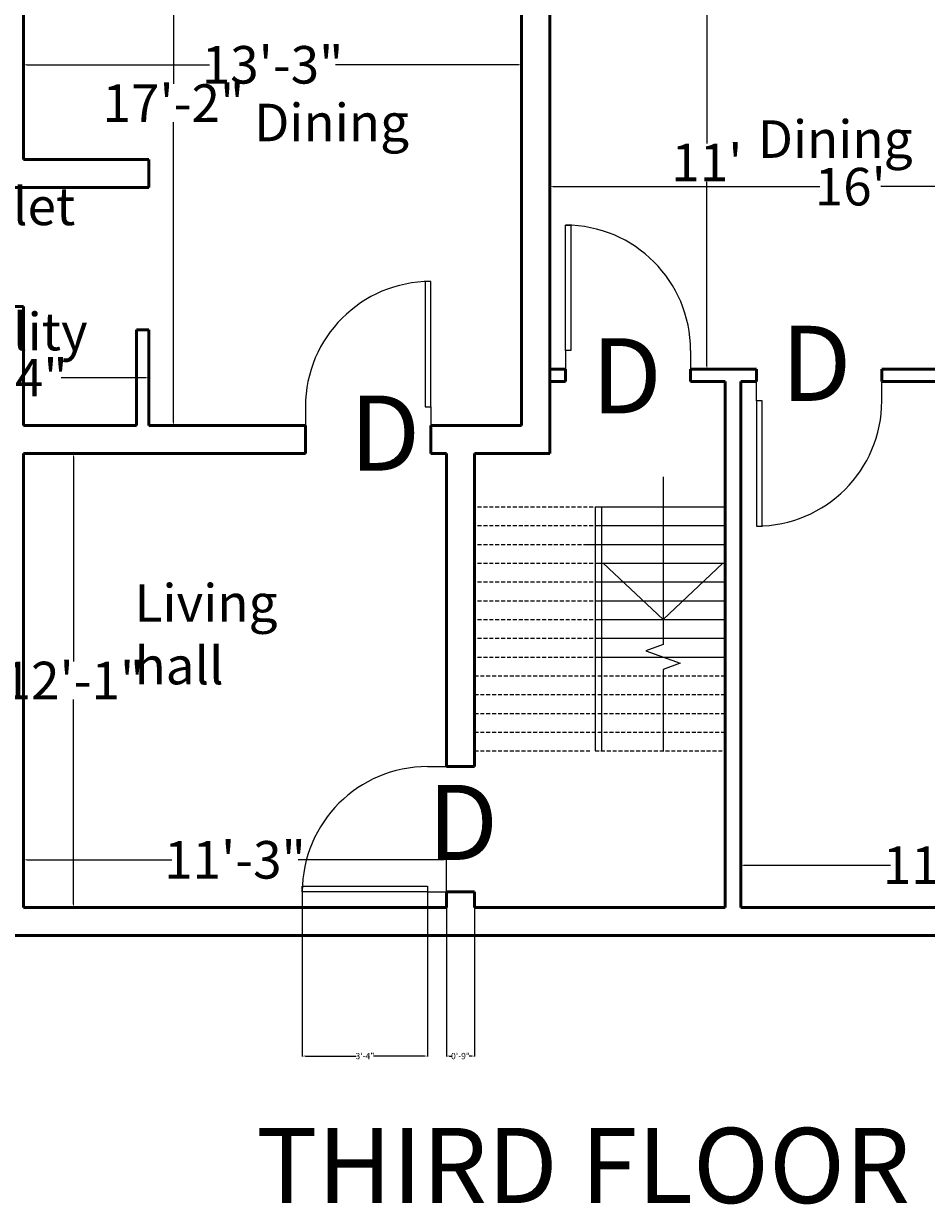
# Model space of a CAD drawing. Units: inches. Extents: x 409 to 7572, y 7 to 725.
# Tile 22 of 38: x 4335 to 4623, y 71 to 448. Entities that reach past the tile are written whole.
import ezdxf

# ---------------------------------------------------------------- set-up
doc = ezdxf.new("R2010")
doc.units = ezdxf.units.IN
doc.header["$MEASUREMENT"] = 0
doc.linetypes.add('HIDDEN', pattern=[0.375, 0.25, -0.125])
for name, color, linetype, lineweight in [('A-ANNO-DIMS', 2, 'Continuous', 18), ('A-ANNO-SYMB', 3, 'Continuous', 25), ('A-ANNO-TEXT', 7, 'Continuous', 35), ('A-AREA-IDEN', 7, 'Continuous', 25), ('A-DOOR', 3, 'Continuous', 25), ('A-FLOR-STRS', 6, 'Continuous', 25), ('A-FLOR-STRS-OVHD', 6, 'HIDDEN', 18), ('A-WALL', 7, 'Continuous', 50)]:
    doc.layers.add(name, color=color, linetype=linetype, lineweight=lineweight)
doc.styles.get("Standard").update_dxf_attribs({"font": 'arial.ttf'})
doc.dimstyles.get("Standard").update_dxf_attribs({"dimtxt": 2, "dimasz": 1, "dimexe": 0.18, "dimexo": 0.0625, "dimgap": 0.09, "dimtad": 0, "dimtih": 1, "dimtoh": 1, "dimdec": 0, "dimzin": 0, "dimdsep": 46, "dimlunit": 3, "dimtxsty": 'Standard', "dimcen": 0.09, "dimadec": 0, "dimazin": 0, "dimtfac": 1, "dimtdec": 0, "dimtofl": 0, "dimtmove": 0, "dimatfit": 3, "dimfxl": 1, "dimtolj": 1, "dimtzin": 0, "dimarcsym": 0})

# ---------------------------------------------------------------- blocks, each defined once
blk = doc.blocks.new('*U2')
for p, q in [((0, 0), (0, -6)), ((-40, 0), (-40, -6))]:
    blk.add_line(p, q)
blk.add_lwpolyline([(0, 0), (0, 40), (-1.75, 40), (-1.75, 0)], close=True)
blk.add_arc((0, 0), 40, 90, 180)
blk = doc.blocks.new('*U3')
for p, q in [((0, 0), (0, -6)), ((40, 0), (40, -6))]:
    blk.add_line(p, q)
blk.add_lwpolyline([(0, 0), (0, 40), (1.75, 40), (1.75, 0)], close=True)
blk.add_arc((0, 0), 40, 0, 90)
blk = doc.blocks.new('*U4')
for p, q in [((0, 0), (0, -6)), ((40, 0), (40, -6))]:
    blk.add_line(p, q)
blk.add_lwpolyline([(0, 0), (0, 40), (1.75, 40), (1.75, 0)], close=True)
blk.add_arc((0, 0), 40, 0, 90)
blk = doc.blocks.new('*U5')
for p, q in [((0, 0), (0, 6)), ((40, 0), (40, 6))]:
    blk.add_line(p, q)
blk.add_lwpolyline([(0, 0), (0, -40), (1.75, -40), (1.75, 0)], close=True)
blk.add_arc((0, 0), 40, 270, 0)
blk = doc.blocks.new('*D96')
at = {"layer": 'A-ANNO-DIMS', "color": 0, "lineweight": -2, "transparency": 16777216}
for p, q in [((4563.94, 165.59), (4563.94, 179.18)), ((4564.94, 179), (4611.8, 179)), ((4698.94, 179), (4652.08, 179)), ((4699.94, 165.59), (4699.94, 179.18))]:
    blk.add_line(p, q, dxfattribs=at)
at = {"layer": 'A-ANNO-DIMS', "color": 0, "transparency": 16777216}
for points in [[(4564.94, 179.16), (4564.94, 178.83), (4563.94, 179)], [(4698.94, 179.16), (4698.94, 178.83), (4699.94, 179)]]:
    blk.add_solid(points, dxfattribs=at)
at = {"layer": 'DEFPOINTS', "color": 0, "transparency": 16777216}
for p in [(4699.94, 179), (4563.94, 165.53), (4699.94, 165.53)]:
    blk.add_point(p, dxfattribs=at)
at = {"layer": 'A-ANNO-DIMS', "color": 0, "transparency": 16777216, "insert": (4631.94, 179), "char_height": 2, "attachment_point": 5}
blk.add_mtext('\\A1;{\\H6x;11\'-4"}', dxfattribs=at)
blk = doc.blocks.new('*D97')
at = {"layer": 'A-ANNO-DIMS', "color": 0, "lineweight": -2, "transparency": 16777216}
for p, q in [((4334.94, 165.59), (4334.94, 180.91)), ((4335.94, 180.73), (4382.3, 180.73)), ((4468.94, 180.73), (4422.58, 180.73)), ((4469.94, 165.59), (4469.94, 180.91))]:
    blk.add_line(p, q, dxfattribs=at)
at = {"layer": 'A-ANNO-DIMS', "color": 0, "transparency": 16777216}
for points in [[(4335.94, 180.9), (4335.94, 180.56), (4334.94, 180.73)], [(4468.94, 180.9), (4468.94, 180.56), (4469.94, 180.73)]]:
    blk.add_solid(points, dxfattribs=at)
at = {"layer": 'DEFPOINTS', "color": 0, "transparency": 16777216}
for p in [(4469.94, 180.73), (4334.94, 165.53), (4469.94, 165.53)]:
    blk.add_point(p, dxfattribs=at)
at = {"layer": 'A-ANNO-DIMS', "color": 0, "transparency": 16777216, "insert": (4402.44, 180.73), "char_height": 2, "attachment_point": 5}
blk.add_mtext('\\A1;{\\H6x;11\'-3"}', dxfattribs=at)
blk = doc.blocks.new('*D98')
at = {"layer": 'A-ANNO-DIMS', "color": 0, "lineweight": -2, "transparency": 16777216}
for p, q in [((4335, 310.53), (4351.04, 310.53)), ((4350.86, 309.53), (4350.86, 244.15)), ((4350.86, 166.53), (4350.86, 231.92)), ((4335, 165.53), (4351.04, 165.53))]:
    blk.add_line(p, q, dxfattribs=at)
at = {"layer": 'A-ANNO-DIMS', "color": 0, "transparency": 16777216}
for points in [[(4350.7, 309.53), (4351.03, 309.53), (4350.86, 310.53)], [(4350.7, 166.53), (4351.03, 166.53), (4350.86, 165.53)]]:
    blk.add_solid(points, dxfattribs=at)
at = {"layer": 'DEFPOINTS', "color": 0, "transparency": 16777216}
for p in [(4334.94, 310.53), (4334.94, 165.53), (4350.86, 165.53)]:
    blk.add_point(p, dxfattribs=at)
at = {"layer": 'A-ANNO-DIMS', "color": 0, "transparency": 16777216, "insert": (4350.86, 238.03), "char_height": 2, "attachment_point": 5}
blk.add_mtext('\\A1;{\\H6x;12\'-1"}', dxfattribs=at)
blk = doc.blocks.new('*D110')
at = {"layer": 'A-ANNO-DIMS', "color": 0, "lineweight": -2, "transparency": 16777216}
for p, q in [((4334.94, 404.59), (4334.94, 434.95)), ((4335.94, 434.77), (4394.3, 434.77)), ((4492.94, 434.77), (4434.58, 434.77)), ((4493.94, 404.59), (4493.94, 434.95))]:
    blk.add_line(p, q, dxfattribs=at)
at = {"layer": 'A-ANNO-DIMS', "color": 0, "transparency": 16777216}
for points in [[(4335.94, 434.93), (4335.94, 434.6), (4334.94, 434.77)], [(4492.94, 434.93), (4492.94, 434.6), (4493.94, 434.77)]]:
    blk.add_solid(points, dxfattribs=at)
at = {"layer": 'DEFPOINTS', "color": 0, "transparency": 16777216}
for p in [(4493.94, 434.77), (4334.94, 404.53), (4493.94, 404.53)]:
    blk.add_point(p, dxfattribs=at)
at = {"layer": 'A-ANNO-DIMS', "color": 0, "transparency": 16777216, "insert": (4414.44, 434.77), "char_height": 2, "attachment_point": 5}
blk.add_mtext('\\A1;{\\H6x;13\'-3"}', dxfattribs=at)
blk = doc.blocks.new('*D111')
at = {"layer": 'A-ANNO-DIMS', "color": 0, "lineweight": -2, "transparency": 16777216}
for p, q in [((4391.88, 525.53), (4382.6, 525.53)), ((4382.78, 524.53), (4382.78, 428.65)), ((4382.78, 320.53), (4382.78, 416.42)), ((4399.88, 319.53), (4382.6, 319.53))]:
    blk.add_line(p, q, dxfattribs=at)
at = {"layer": 'A-ANNO-DIMS', "color": 0, "transparency": 16777216}
for points in [[(4382.61, 524.53), (4382.94, 524.53), (4382.78, 525.53)], [(4382.61, 320.53), (4382.94, 320.53), (4382.78, 319.53)]]:
    blk.add_solid(points, dxfattribs=at)
at = {"layer": 'DEFPOINTS', "color": 0, "transparency": 16777216}
for p in [(4391.94, 525.53), (4382.78, 319.53), (4399.94, 319.53)]:
    blk.add_point(p, dxfattribs=at)
at = {"layer": 'A-ANNO-DIMS', "color": 0, "transparency": 16777216, "insert": (4382.78, 422.53), "char_height": 2, "attachment_point": 5}
blk.add_mtext('\\A1;{\\H6x;17\'-2"}', dxfattribs=at)
blk = doc.blocks.new('*D108')
at = {"layer": 'A-ANNO-DIMS', "color": 0, "lineweight": -2, "transparency": 16777216}
for p, q in [((4502.94, 403.47), (4502.94, 395.65)), ((4694.94, 403.47), (4694.94, 395.65)), ((4503.94, 395.83), (4589.23, 395.83)), ((4693.94, 395.83), (4608.65, 395.83))]:
    blk.add_line(p, q, dxfattribs=at)
at = {"layer": 'A-ANNO-DIMS', "color": 0, "transparency": 16777216}
for points in [[(4503.94, 396), (4503.94, 395.66), (4502.94, 395.83)], [(4693.94, 396), (4693.94, 395.66), (4694.94, 395.83)]]:
    blk.add_solid(points, dxfattribs=at)
at = {"layer": 'DEFPOINTS', "color": 0, "transparency": 16777216}
for p in [(4502.94, 403.53), (4694.94, 403.53), (4694.94, 395.83)]:
    blk.add_point(p, dxfattribs=at)
at = {"layer": 'A-ANNO-DIMS', "color": 0, "transparency": 16777216, "insert": (4598.94, 395.83), "char_height": 2, "attachment_point": 5}
blk.add_mtext("\\A1;{\\H6x;16'}", dxfattribs=at)
blk = doc.blocks.new('*D112')
at = {"layer": 'A-ANNO-DIMS', "color": 0, "lineweight": -2, "transparency": 16777216}
for p, q in [((4557.2, 469.53), (4552.96, 469.53)), ((4553.14, 468.53), (4553.14, 409.65)), ((4553.14, 338.53), (4553.14, 397.42)), ((4558.38, 337.53), (4552.96, 337.53))]:
    blk.add_line(p, q, dxfattribs=at)
at = {"layer": 'A-ANNO-DIMS', "color": 0, "transparency": 16777216}
for points in [[(4552.97, 468.53), (4553.31, 468.53), (4553.14, 469.53)], [(4552.97, 338.53), (4553.31, 338.53), (4553.14, 337.53)]]:
    blk.add_solid(points, dxfattribs=at)
at = {"layer": 'DEFPOINTS', "color": 0, "transparency": 16777216}
for p in [(4557.27, 469.53), (4553.14, 337.53), (4558.44, 337.53)]:
    blk.add_point(p, dxfattribs=at)
at = {"layer": 'A-ANNO-DIMS', "color": 0, "transparency": 16777216, "insert": (4553.14, 403.53), "char_height": 2, "attachment_point": 5}
blk.add_mtext("\\A1;{\\H6x;11'}", dxfattribs=at)
blk = doc.blocks.new('*D117')
at = {"layer": 'A-ANNO-DIMS', "color": 0, "lineweight": -2, "transparency": 16777216}
for p, q in [((4286.94, 346.33), (4286.94, 334.6)), ((4374.94, 346.33), (4374.94, 334.6)), ((4287.94, 334.78), (4314.95, 334.78)), ((4373.94, 334.78), (4346.93, 334.78))]:
    blk.add_line(p, q, dxfattribs=at)
at = {"layer": 'A-ANNO-DIMS', "color": 0, "transparency": 16777216}
for points in [[(4287.94, 334.95), (4287.94, 334.61), (4286.94, 334.78)], [(4373.94, 334.95), (4373.94, 334.61), (4374.94, 334.78)]]:
    blk.add_solid(points, dxfattribs=at)
at = {"layer": 'DEFPOINTS', "color": 0, "transparency": 16777216}
for p in [(4286.94, 346.39), (4374.94, 346.39), (4374.94, 334.78)]:
    blk.add_point(p, dxfattribs=at)
at = {"layer": 'A-ANNO-DIMS', "color": 0, "transparency": 16777216, "insert": (4330.94, 334.78), "char_height": 2, "attachment_point": 5}
blk.add_mtext('\\A1;{\\H6x;7\'-4"}', dxfattribs=at)
blk = doc.blocks.new('*D189')
at = {"layer": 'A-ANNO-DIMS', "color": 0, "lineweight": -2, "transparency": 16777216}
for p, q in [((4469.94, 165.47), (4469.94, 117.85)), ((4478.94, 165.47), (4478.94, 117.85)), ((4470.94, 118.03), (4471.69, 118.03)), ((4477.94, 118.03), (4477.19, 118.03))]:
    blk.add_line(p, q, dxfattribs=at)
at = {"layer": 'A-ANNO-DIMS', "color": 0, "transparency": 16777216}
for points in [[(4470.94, 118.2), (4470.94, 117.86), (4469.94, 118.03)], [(4477.94, 118.2), (4477.94, 117.86), (4478.94, 118.03)]]:
    blk.add_solid(points, dxfattribs=at)
at = {"layer": 'DEFPOINTS', "color": 0, "transparency": 16777216}
for p in [(4469.94, 165.53), (4478.94, 165.53), (4478.94, 118.03)]:
    blk.add_point(p, dxfattribs=at)
at = {"layer": 'A-ANNO-DIMS', "color": 0, "transparency": 16777216, "insert": (4474.44, 118.03), "char_height": 2, "attachment_point": 5}
blk.add_mtext('\\A1;0\'-9"', dxfattribs=at)
blk = doc.blocks.new('*D191')
at = {"layer": 'A-ANNO-DIMS', "color": 0, "lineweight": -2, "transparency": 16777216}
for p, q in [((4423.94, 170.47), (4423.94, 117.85)), ((4463.94, 170.47), (4463.94, 117.85)), ((4424.94, 118.03), (4441.19, 118.03)), ((4462.94, 118.03), (4446.69, 118.03))]:
    blk.add_line(p, q, dxfattribs=at)
at = {"layer": 'A-ANNO-DIMS', "color": 0, "transparency": 16777216}
for points in [[(4424.94, 118.2), (4424.94, 117.86), (4423.94, 118.03)], [(4462.94, 118.2), (4462.94, 117.86), (4463.94, 118.03)]]:
    blk.add_solid(points, dxfattribs=at)
at = {"layer": 'DEFPOINTS', "color": 0, "transparency": 16777216}
for p in [(4423.94, 170.53), (4463.94, 170.53), (4463.94, 118.03)]:
    blk.add_point(p, dxfattribs=at)
at = {"layer": 'A-ANNO-DIMS', "color": 0, "transparency": 16777216, "insert": (4443.94, 118.03), "char_height": 2, "attachment_point": 5}
blk.add_mtext('\\A1;3\'-4"', dxfattribs=at)

msp = doc.modelspace()

# ---------------------------------------------------------------- linework, layer by layer
at = {"layer": 'A-FLOR-STRS'}
for p, q in [((4539.15, 303.06), (4539.15, 257.53)), ((4517.44, 293.53), (4558.94, 293.53)), ((4517.44, 293.53), (4517.44, 215.53)), ((4519.44, 293.53), (4519.44, 215.53)), ((4517.44, 287.53), (4558.94, 287.53)), ((4514.6, 281.53), (4558.94, 281.53)), ((4517.44, 275.53), (4558.94, 275.53)), ((4539.15, 257.53), (4520.02, 275.53)), ((4539.15, 257.53), (4558.27, 275.53)), ((4517.44, 269.53), (4558.94, 269.53)), ((4517.44, 263.53), (4558.94, 263.53)), ((4517.44, 257.53), (4558.94, 257.53)), ((4517.44, 251.53), (4558.94, 251.53)), ((4517.44, 245.53), (4558.94, 245.53))]:
    msp.add_line(p, q, dxfattribs=at)
msp.add_lwpolyline([(4539.15, 257.71), (4539.15, 249.53), (4533.65, 247.53), (4544.64, 243.53), (4539.15, 241.53), (4539.15, 215.35)], dxfattribs=at)
at = {"layer": 'A-FLOR-STRS-OVHD', "ltscale": 5}
for p, q in [((4479.94, 293.53), (4517.44, 293.53)), ((4479.94, 287.53), (4517.44, 287.53)), ((4479.94, 281.53), (4514.6, 281.53)), ((4479.94, 275.53), (4517.44, 275.53)), ((4479.94, 269.53), (4517.44, 269.53)), ((4479.94, 263.53), (4517.44, 263.53)), ((4479.94, 257.53), (4517.44, 257.53)), ((4479.94, 251.53), (4517.44, 251.53)), ((4479.94, 245.53), (4517.44, 245.53)), ((4478.94, 239.53), (4558.94, 239.53)), ((4478.94, 233.53), (4558.94, 233.53)), ((4478.94, 227.53), (4558.94, 227.53)), ((4478.94, 221.53), (4558.94, 221.53)), ((4478.94, 215.53), (4516.44, 215.53)), ((4517.44, 215.53), (4558.94, 215.53))]:
    msp.add_line(p, q, dxfattribs=at)
at = {"layer": 'A-WALL'}
for p, q in [((4334.94, 525.53), (4334.94, 404.53)), ((4493.94, 525.53), (4493.94, 319.53)), ((4502.94, 469.53), (4502.94, 337.53)), ((4374.94, 404.53), (4334.94, 404.53)), ((4374.94, 404.53), (4374.94, 395.53)), ((4334.94, 395.53), (4286.94, 395.53)), ((4374.94, 395.53), (4334.94, 395.53)), ((4334.94, 357.53), (4325.94, 357.53)), ((4334.94, 357.53), (4334.94, 319.53)), ((4370.94, 350.03), (4370.94, 319.53)), ((4374.94, 350.03), (4370.94, 350.03)), ((4374.94, 350.03), (4374.94, 319.53)), ((4502.94, 337.53), (4507.94, 337.53)), ((4502.94, 337.53), (4502.94, 333.53)), ((4507.94, 337.53), (4507.94, 333.53)), ((4547.94, 337.53), (4568.94, 337.53)), ((4547.94, 337.53), (4547.94, 333.53)), ((4568.94, 333.53), (4568.94, 337.53)), ((4609, 337.53), (4694.94, 337.53)), ((4609, 337.53), (4609, 333.53)), ((4502.94, 333.53), (4507.94, 333.53)), ((4502.94, 333.53), (4502.94, 310.53)), ((4547.94, 333.53), (4558.94, 333.53)), ((4558.94, 333.53), (4558.94, 165.53)), ((4563.94, 333.53), (4568.94, 333.53)), ((4563.94, 333.53), (4563.94, 165.53)), ((4609, 333.53), (4694.94, 333.53)), ((4370.94, 319.53), (4334.94, 319.53)), ((4424.94, 319.53), (4374.94, 319.53)), ((4424.94, 319.53), (4424.94, 310.53)), ((4493.94, 319.53), (4464.94, 319.53)), ((4464.94, 310.53), (4464.94, 319.53)), ((4424.94, 310.53), (4334.94, 310.53)), ((4334.94, 310.53), (4334.94, 165.53)), ((4469.94, 310.53), (4464.94, 310.53)), ((4469.94, 310.53), (4469.94, 210.53)), ((4502.94, 310.53), (4478.94, 310.53)), ((4478.94, 310.53), (4478.94, 210.53)), ((4469.94, 210.53), (4478.94, 210.53)), ((4469.94, 170.53), (4469.94, 165.53)), ((4478.94, 170.53), (4469.94, 170.53)), ((4478.94, 170.53), (4478.94, 165.53)), ((4334.94, 165.53), (4469.94, 165.53)), ((4478.94, 165.53), (4558.94, 165.53)), ((4563.94, 165.53), (4699.94, 165.53)), ((4325.94, 156.53), (4699.94, 156.53))]:
    msp.add_line(p, q, dxfattribs=at)

# ---------------------------------------------------------------- block references
at = {"layer": 'A-DOOR'}
for name, p in [('*U4', (4507.94, 343.53)), ('*U2', (4464.94, 325.53)), ('*U5', (4569, 327.37))]:
    msp.add_blockref(name, p, dxfattribs=at)
at = {"layer": 'A-DOOR', "rotation": 90}
msp.add_blockref('*U3', (4463.94, 170.53), dxfattribs=at)

# ---------------------------------------------------------------- texts
at = {"layer": 'A-ANNO-SYMB', "char_height": 24, "attachment_point": 1}
for insert in [(4576.77, 351.37), (4516.24, 347.4), (4439.08, 329.09), (4463.94, 204.69)]:
    msp.add_mtext_dynamic_manual_height_columns('D', width=19.1972, gutter_width=1, heights=[0], dxfattribs=dict(at, insert=insert))
at = {"layer": 'A-ANNO-TEXT', "insert": (4409.15, 95.06), "char_height": 24, "attachment_point": 1}
msp.add_mtext_dynamic_manual_height_columns('THIRD FLOOR', width=577.2242, gutter_width=1, heights=[0], dxfattribs=at)
at = {"layer": 'A-AREA-IDEN', "char_height": 12, "attachment_point": 1}
for s, width, insert in [('Dining ', 67.5069, (4408.55, 422.33)), ('Dining ', 67.5069, (4569.37, 417.03)), ('toilet / utility', 49.2946, (4310.94, 395.53)), ('Living hall', 58.8843, (4370.37, 268.81))]:
    msp.add_mtext_dynamic_manual_height_columns(s, width=width, gutter_width=1, heights=[0], dxfattribs=dict(at, insert=insert))

# ---------------------------------------------------------------- dimensions: what is measured, and where the dimension line sits
at = {"layer": 'A-ANNO-DIMS'}
dim = msp.add_linear_dim(base=(4382.78, 319.53), p1=(4391.94, 525.53), p2=(4399.94, 319.53), angle=90, text='{\\H6x;<>}', dimstyle='Standard', override={"dimclrd": 0, "dimclre": 0, "dimclrt": 0}, dxfattribs=at)
dim.commit()
dim.dimension.update_dxf_attribs({"geometry": '*D111', "text_midpoint": (4382.78, 422.53), "dimtype": 160})
for base, p1, p2, picture, middle in [((4553.14, 337.53), (4557.27, 469.53), (4558.44, 337.53), '*D112', (4553.14, 403.53)), ((4350.86, 165.53), (4334.94, 310.53), (4334.94, 165.53), '*D98', (4350.86, 238.03))]:
    dim = msp.add_linear_dim(base=base, p1=p1, p2=p2, angle=90, text='{\\H6x;<>}', dimstyle='Standard', override={"dimclrd": 0, "dimclre": 0, "dimclrt": 0}, dxfattribs=at)
    dim.commit()
    dim.dimension.update_dxf_attribs({"geometry": picture, "text_midpoint": middle})
for base, p1, p2, picture, middle in [((4493.94, 434.77), (4334.94, 404.53), (4493.94, 404.53), '*D110', (4414.44, 434.77)), ((4374.94, 334.78), (4286.94, 346.39), (4374.94, 346.39), '*D117', (4330.94, 334.78)), ((4469.94, 180.73), (4334.94, 165.53), (4469.94, 165.53), '*D97', (4402.44, 180.73)), ((4699.94, 179), (4563.94, 165.53), (4699.94, 165.53), '*D96', (4631.94, 179))]:
    dim = msp.add_linear_dim(base=base, p1=p1, p2=p2, text='{\\H6x;<>}', dimstyle='Standard', override={"dimclrd": 0, "dimclre": 0, "dimclrt": 0}, dxfattribs=at)
    dim.commit()
    dim.dimension.update_dxf_attribs({"geometry": picture, "text_midpoint": middle})
dim = msp.add_linear_dim(base=(4694.94, 395.83), p1=(4502.94, 403.53), p2=(4694.94, 403.53), text='{\\H6x;<>}', dimstyle='Standard', override={"dimclrd": 0, "dimclre": 0, "dimclrt": 0}, dxfattribs=at)
dim.commit()
dim.dimension.update_dxf_attribs({"geometry": '*D108', "text_midpoint": (4598.94, 395.83), "dimtype": 160})
for base, p1, p2, picture, middle in [((4463.94, 118.03), (4423.94, 170.53), (4463.94, 170.53), '*D191', (4443.94, 118.03)), ((4478.94, 118.03), (4469.94, 165.53), (4478.94, 165.53), '*D189', (4474.44, 118.03))]:
    dim = msp.add_linear_dim(base=base, p1=p1, p2=p2, dimstyle='Standard', override={"dimdec": 1, "dimlfac": 1, "dimrnd": 0, "dimzin": 1, "dimdsep": 46, "dimlunit": 4, "dimfrac": 2}, dxfattribs=at)
    dim.commit()
    dim.dimension.update_dxf_attribs({"geometry": picture, "text_midpoint": middle})

doc.saveas('drawing.dxf')
